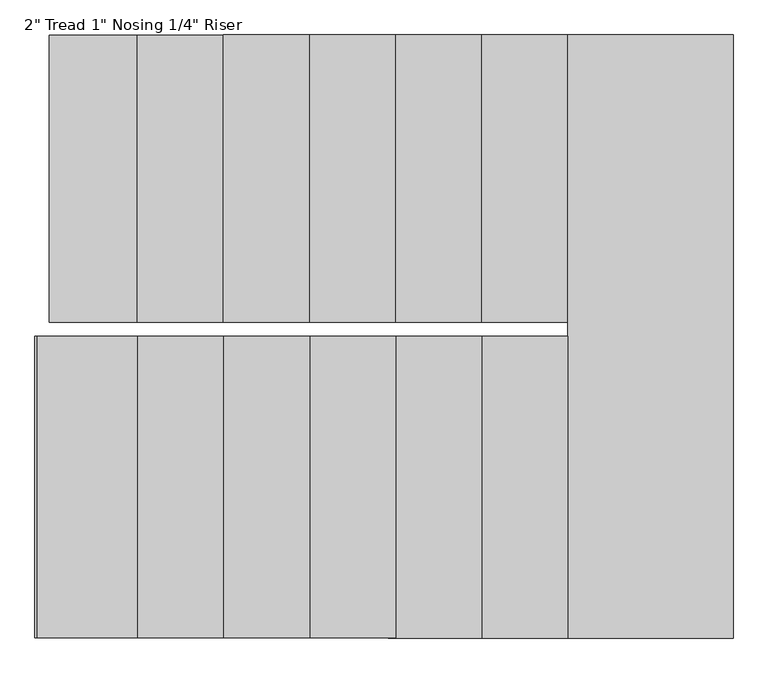
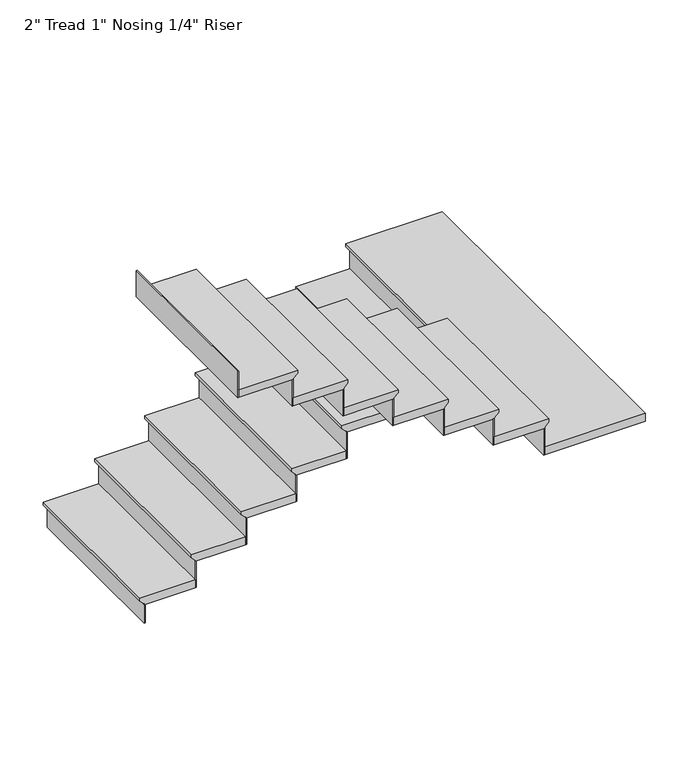
"""IFC4 building model written with IfcOpenShell, lengths in millimetres: stair flight geometry."""

from ifc_helpers import new_model, si_unit, origin, place, context, project, spatial, faceted_brep, source, transform, mapped, element, save


def stair_flight_c67f7d23(model_context):
    return source(origin(), model_context, "Body", "Brep", [
        faceted_brep([(-1167.6638307, -167.7482799, 6551.0833333), (-1167.6638307, -167.7482799, 6570.1333333), (-1167.6638307, 848.2517201, 6570.1333333), (-1167.6638307, 848.2517201, 6551.0833333), (-1142.2638307, -167.7482799, 6525.6833333), (-1142.2638307, 848.2517201, 6525.6833333), (-831.1138307, -167.7482799, 6570.1333333), (-831.1138307, 848.2517201, 6570.1333333), (-1142.2638307, 848.2517201, 6519.3333333), (-831.1138307, 848.2517201, 6519.3333333), (-831.1138307, -167.7482799, 6519.3333333), (-1142.2638307, -167.7482799, 6519.3333333)], [[[0, 1, 2, 3]], [[4, 0, 3, 5]], [[2, 1, 6, 7]], [[8, 9, 10, 11]], [[2, 7, 9, 8, 5, 3]], [[8, 11, 4, 5]], [[6, 1, 0, 4, 11, 10]], [[7, 6, 10, 9]]]),
        faceted_brep([(-1142.2638307, -167.7482799, 6519.3333333), (-1142.2638307, -167.7482799, 6400.8), (-1135.9138307, -167.7482799, 6400.8), (-1135.9138307, -167.7482799, 6519.3333333), (-1142.2638307, 848.2517201, 6519.3333333), (-1135.9138307, 848.2517201, 6519.3333333), (-1135.9138307, 848.2517201, 6400.8), (-1142.2638307, 848.2517201, 6400.8)], [[[0, 1, 2, 3]], [[4, 5, 6, 7]], [[1, 0, 4, 7]], [[2, 1, 7, 6]], [[3, 2, 6, 5]], [[0, 3, 5, 4]]]),
        faceted_brep([(-831.1138307, -167.7482799, 6688.6666667), (-831.1138307, -167.7482799, 6519.3333333), (-824.7638307, -167.7482799, 6519.3333333), (-824.7638307, -167.7482799, 6688.6666667), (-831.1138307, 848.2517201, 6688.6666667), (-824.7638307, 848.2517201, 6688.6666667), (-824.7638307, 848.2517201, 6519.3333333), (-831.1138307, 848.2517201, 6519.3333333)], [[[0, 1, 2, 3]], [[4, 5, 6, 7]], [[1, 0, 4, 7]], [[2, 1, 7, 6]], [[3, 2, 6, 5]], [[0, 3, 5, 4]]]),
        faceted_brep([(-856.5138307, 848.2517201, 6739.4666667), (-856.5138307, -167.7482799, 6739.4666667), (-526.3138307, -167.7482799, 6739.4666667), (-526.3138307, 848.2517201, 6739.4666667), (-831.1138307, 848.2517201, 6688.6666667), (-526.3138307, 848.2517201, 6688.6666667), (-526.3138307, -167.7482799, 6688.6666667), (-831.1138307, -167.7482799, 6688.6666667), (-831.1138307, 848.2517201, 6695.0166667), (-856.5138307, 848.2517201, 6720.4166667), (-831.1138307, -167.7482799, 6695.0166667), (-856.5138307, -167.7482799, 6720.4166667)], [[[0, 1, 2, 3]], [[4, 5, 6, 7]], [[0, 3, 5, 4, 8, 9]], [[4, 7, 10, 8]], [[2, 1, 11, 10, 7, 6]], [[3, 2, 6, 5]], [[11, 1, 0, 9]], [[10, 11, 9, 8]]]),
        faceted_brep([(-526.3138307, -167.7482799, 6858.0), (-526.3138307, -167.7482799, 6688.6666667), (-519.9638307, -167.7482799, 6688.6666667), (-519.9638307, -167.7482799, 6858.0), (-526.3138307, 848.2517201, 6858.0), (-519.9638307, 848.2517201, 6858.0), (-519.9638307, 848.2517201, 6688.6666667), (-526.3138307, 848.2517201, 6688.6666667)], [[[0, 1, 2, 3]], [[4, 5, 6, 7]], [[1, 0, 4, 7]], [[2, 1, 7, 6]], [[3, 2, 6, 5]], [[0, 3, 5, 4]]]),
        faceted_brep([(-551.7138307, 848.2517201, 6908.8), (-551.7138307, -167.7482799, 6908.8), (-221.5138307, -167.7482799, 6908.8), (-221.5138307, 848.2517201, 6908.8), (-526.3138307, 848.2517201, 6858.0), (-221.5138307, 848.2517201, 6858.0), (-221.5138307, -167.7482799, 6858.0), (-526.3138307, -167.7482799, 6858.0), (-526.3138307, 848.2517201, 6864.35), (-551.7138307, 848.2517201, 6889.75), (-526.3138307, -167.7482799, 6864.35), (-551.7138307, -167.7482799, 6889.75)], [[[0, 1, 2, 3]], [[4, 5, 6, 7]], [[0, 3, 5, 4, 8, 9]], [[4, 7, 10, 8]], [[2, 1, 11, 10, 7, 6]], [[3, 2, 6, 5]], [[11, 1, 0, 9]], [[10, 11, 9, 8]]]),
        faceted_brep([(-221.5138307, -167.7482799, 7027.3333333), (-221.5138307, -167.7482799, 6858.0), (-215.1638307, -167.7482799, 6858.0), (-215.1638307, -167.7482799, 7027.3333333), (-221.5138307, 848.2517201, 7027.3333333), (-215.1638307, 848.2517201, 7027.3333333), (-215.1638307, 848.2517201, 6858.0), (-221.5138307, 848.2517201, 6858.0)], [[[0, 1, 2, 3]], [[4, 5, 6, 7]], [[1, 0, 4, 7]], [[2, 1, 7, 6]], [[3, 2, 6, 5]], [[0, 3, 5, 4]]]),
        faceted_brep([(-246.9138307, 848.2517201, 7078.1333333), (-246.9138307, -167.7482799, 7078.1333333), (83.2861693, -167.7482799, 7078.1333333), (83.2861693, 848.2517201, 7078.1333333), (-221.5138307, 848.2517201, 7027.3333333), (83.2861693, 848.2517201, 7027.3333333), (83.2861693, -167.7482799, 7027.3333333), (-221.5138307, -167.7482799, 7027.3333333), (-221.5138307, 848.2517201, 7033.6833333), (-246.9138307, 848.2517201, 7059.0833333), (-221.5138307, -167.7482799, 7033.6833333), (-246.9138307, -167.7482799, 7059.0833333)], [[[0, 1, 2, 3]], [[4, 5, 6, 7]], [[0, 3, 5, 4, 8, 9]], [[4, 7, 10, 8]], [[2, 1, 11, 10, 7, 6]], [[3, 2, 6, 5]], [[11, 1, 0, 9]], [[10, 11, 9, 8]]]),
        faceted_brep([(83.2861693, -167.7482799, 7196.6666667), (83.2861693, -167.7482799, 7027.3333333), (89.6361693, -167.7482799, 7027.3333333), (89.6361693, -167.7482799, 7196.6666667), (83.2861693, 848.2517201, 7196.6666667), (89.6361693, 848.2517201, 7196.6666667), (89.6361693, 848.2517201, 7027.3333333), (83.2861693, 848.2517201, 7027.3333333)], [[[0, 1, 2, 3]], [[4, 5, 6, 7]], [[1, 0, 4, 7]], [[2, 1, 7, 6]], [[3, 2, 6, 5]], [[0, 3, 5, 4]]]),
        faceted_brep([(57.8861693, 848.2517201, 7247.4666667), (57.8861693, -167.7482799, 7247.4666667), (388.0861693, -167.7482799, 7247.4666667), (388.0861693, 848.2517201, 7247.4666667), (83.2861693, 848.2517201, 7196.6666667), (388.0861693, 848.2517201, 7196.6666667), (388.0861693, -167.7482799, 7196.6666667), (83.2861693, -167.7482799, 7196.6666667), (83.2861693, 848.2517201, 7203.0166667), (57.8861693, 848.2517201, 7228.4166667), (83.2861693, -167.7482799, 7203.0166667), (57.8861693, -167.7482799, 7228.4166667)], [[[0, 1, 2, 3]], [[4, 5, 6, 7]], [[0, 3, 5, 4, 8, 9]], [[4, 7, 10, 8]], [[2, 1, 11, 10, 7, 6]], [[3, 2, 6, 5]], [[11, 1, 0, 9]], [[10, 11, 9, 8]]]),
        faceted_brep([(388.0861693, -167.7482799, 7366.0), (388.0861693, -167.7482799, 7196.6666667), (394.4361693, -167.7482799, 7196.6666667), (394.4361693, -167.7482799, 7366.0), (388.0861693, 848.2517201, 7366.0), (394.4361693, 848.2517201, 7366.0), (394.4361693, 848.2517201, 7196.6666667), (388.0861693, 848.2517201, 7196.6666667)], [[[0, 1, 2, 3]], [[4, 5, 6, 7]], [[1, 0, 4, 7]], [[2, 1, 7, 6]], [[3, 2, 6, 5]], [[0, 3, 5, 4]]]),
        faceted_brep([(362.6861693, 848.2517201, 7416.8), (362.6861693, -167.7482799, 7416.8), (692.8861693, -167.7482799, 7416.8), (692.8861693, 848.2517201, 7416.8), (388.0861693, 848.2517201, 7366.0), (692.8861693, 848.2517201, 7366.0), (692.8861693, -167.7482799, 7366.0), (388.0861693, -167.7482799, 7366.0), (388.0861693, 848.2517201, 7372.35), (362.6861693, 848.2517201, 7397.75), (388.0861693, -167.7482799, 7372.35), (362.6861693, -167.7482799, 7397.75)], [[[0, 1, 2, 3]], [[4, 5, 6, 7]], [[0, 3, 5, 4, 8, 9]], [[4, 7, 10, 8]], [[2, 1, 11, 10, 7, 6]], [[3, 2, 6, 5]], [[11, 1, 0, 9]], [[10, 11, 9, 8]]]),
        faceted_brep([(692.8861693, -167.7482799, 7535.3333333), (692.8861693, -167.7482799, 7366.0), (699.2361693, -167.7482799, 7366.0), (699.2361693, -167.7482799, 7535.3333333), (692.8861693, 848.2517201, 7535.3333333), (699.2361693, 848.2517201, 7535.3333333), (699.2361693, 848.2517201, 7366.0), (692.8861693, 848.2517201, 7366.0)], [[[0, 1, 2, 3]], [[4, 5, 6, 7]], [[1, 0, 4, 7]], [[2, 1, 7, 6]], [[3, 2, 6, 5]], [[0, 3, 5, 4]]]),
        faceted_brep([(642.0861693, -1285.3482799, 7586.1333333), (1251.6861693, -1285.3482799, 7586.1333333), (1251.6861693, 848.2517201, 7586.1333333), (667.4861693, 848.2517201, 7586.1333333), (667.4861693, -218.5482799, 7586.1333333), (642.0861693, -218.5482799, 7586.1333333), (1251.6861693, -1285.3482799, 7535.3333333), (642.0861693, -1285.3482799, 7535.3333333), (642.0861693, -218.5482799, 7535.3333333), (667.4861693, -218.5482799, 7535.3333333), (667.4861693, -167.7482799, 7535.3333333), (692.8861693, -167.7482799, 7535.3333333), (692.8861693, 848.2517201, 7535.3333333), (1251.6861693, 848.2517201, 7535.3333333), (692.8861693, 848.2517201, 7541.6833333), (667.4861693, 848.2517201, 7567.0833333), (692.8861693, -167.7482799, 7541.6833333), (667.4861693, -167.7482799, 7567.0833333)], [[[0, 1, 2, 3, 4, 5]], [[6, 7, 8, 9, 10, 11, 12, 13]], [[1, 0, 7, 6]], [[2, 1, 6, 13]], [[3, 2, 13, 12, 14, 15]], [[12, 11, 16, 14]], [[11, 10, 17, 16]], [[4, 3, 15, 17, 10, 9]], [[5, 4, 9, 8]], [[0, 5, 8, 7]], [[15, 14, 16, 17]]]),
        faceted_brep([(642.0861693, -218.5482799, 7704.6666667), (642.0861693, -218.5482799, 7535.3333333), (635.7361693, -218.5482799, 7535.3333333), (635.7361693, -218.5482799, 7704.6666667), (642.0861693, -1285.3482799, 7704.6666667), (635.7361693, -1285.3482799, 7704.6666667), (635.7361693, -1285.3482799, 7535.3333333), (642.0861693, -1285.3482799, 7535.3333333)], [[[0, 1, 2, 3]], [[4, 5, 6, 7]], [[1, 0, 4, 7]], [[2, 1, 7, 6]], [[3, 2, 6, 5]], [[0, 3, 5, 4]]]),
        faceted_brep([(667.4861693, -1285.3482799, 7755.4666667), (667.4861693, -218.5482799, 7755.4666667), (337.2861693, -218.5482799, 7755.4666667), (337.2861693, -1285.3482799, 7755.4666667), (642.0861693, -1285.3482799, 7704.6666667), (337.2861693, -1285.3482799, 7704.6666667), (337.2861693, -218.5482799, 7704.6666667), (642.0861693, -218.5482799, 7704.6666667), (642.0861693, -1285.3482799, 7711.0166667), (667.4861693, -1285.3482799, 7736.4166667), (642.0861693, -218.5482799, 7711.0166667), (667.4861693, -218.5482799, 7736.4166667)], [[[0, 1, 2, 3]], [[4, 5, 6, 7]], [[0, 3, 5, 4, 8, 9]], [[4, 7, 10, 8]], [[2, 1, 11, 10, 7, 6]], [[3, 2, 6, 5]], [[11, 1, 0, 9]], [[10, 11, 9, 8]]]),
        faceted_brep([(337.2861693, -218.5482799, 7874.0), (337.2861693, -218.5482799, 7704.6666667), (330.9361693, -218.5482799, 7704.6666667), (330.9361693, -218.5482799, 7874.0), (337.2861693, -1285.3482799, 7874.0), (330.9361693, -1285.3482799, 7874.0), (330.9361693, -1285.3482799, 7704.6666667), (337.2861693, -1285.3482799, 7704.6666667)], [[[0, 1, 2, 3]], [[4, 5, 6, 7]], [[1, 0, 4, 7]], [[2, 1, 7, 6]], [[3, 2, 6, 5]], [[0, 3, 5, 4]]]),
        faceted_brep([(362.6861693, -1285.3482799, 7924.8), (362.6861693, -218.5482799, 7924.8), (32.4861693, -218.5482799, 7924.8), (32.4861693, -1285.3482799, 7924.8), (337.2861693, -1285.3482799, 7874.0), (32.4861693, -1285.3482799, 7874.0), (32.4861693, -218.5482799, 7874.0), (337.2861693, -218.5482799, 7874.0), (337.2861693, -1285.3482799, 7880.35), (362.6861693, -1285.3482799, 7905.75), (337.2861693, -218.5482799, 7880.35), (362.6861693, -218.5482799, 7905.75)], [[[0, 1, 2, 3]], [[4, 5, 6, 7]], [[0, 3, 5, 4, 8, 9]], [[4, 7, 10, 8]], [[2, 1, 11, 10, 7, 6]], [[3, 2, 6, 5]], [[11, 1, 0, 9]], [[10, 11, 9, 8]]]),
        faceted_brep([(32.4861693, -218.5482799, 8043.3333333), (32.4861693, -218.5482799, 7874.0), (26.1361693, -218.5482799, 7874.0), (26.1361693, -218.5482799, 8043.3333333), (32.4861693, -1285.3482799, 8043.3333333), (26.1361693, -1285.3482799, 8043.3333333), (26.1361693, -1285.3482799, 7874.0), (32.4861693, -1285.3482799, 7874.0)], [[[0, 1, 2, 3]], [[4, 5, 6, 7]], [[1, 0, 4, 7]], [[2, 1, 7, 6]], [[3, 2, 6, 5]], [[0, 3, 5, 4]]]),
        faceted_brep([(57.8861693, -1285.3482799, 8094.1333333), (57.8861693, -218.5482799, 8094.1333333), (-272.3138307, -218.5482799, 8094.1333333), (-272.3138307, -1285.3482799, 8094.1333333), (32.4861693, -1285.3482799, 8043.3333333), (-272.3138307, -1285.3482799, 8043.3333333), (-272.3138307, -218.5482799, 8043.3333333), (32.4861693, -218.5482799, 8043.3333333), (32.4861693, -1285.3482799, 8049.6833333), (57.8861693, -1285.3482799, 8075.0833333), (32.4861693, -218.5482799, 8049.6833333), (57.8861693, -218.5482799, 8075.0833333)], [[[0, 1, 2, 3]], [[4, 5, 6, 7]], [[0, 3, 5, 4, 8, 9]], [[4, 7, 10, 8]], [[2, 1, 11, 10, 7, 6]], [[3, 2, 6, 5]], [[11, 1, 0, 9]], [[10, 11, 9, 8]]]),
        faceted_brep([(-272.3138307, -218.5482799, 8212.6666667), (-272.3138307, -218.5482799, 8043.3333333), (-278.6638307, -218.5482799, 8043.3333333), (-278.6638307, -218.5482799, 8212.6666667), (-272.3138307, -1285.3482799, 8212.6666667), (-278.6638307, -1285.3482799, 8212.6666667), (-278.6638307, -1285.3482799, 8043.3333333), (-272.3138307, -1285.3482799, 8043.3333333)], [[[0, 1, 2, 3]], [[4, 5, 6, 7]], [[1, 0, 4, 7]], [[2, 1, 7, 6]], [[3, 2, 6, 5]], [[0, 3, 5, 4]]]),
        faceted_brep([(-246.9138307, -1285.3482799, 8263.4666667), (-246.9138307, -218.5482799, 8263.4666667), (-577.1138307, -218.5482799, 8263.4666667), (-577.1138307, -1285.3482799, 8263.4666667), (-272.3138307, -1285.3482799, 8212.6666667), (-577.1138307, -1285.3482799, 8212.6666667), (-577.1138307, -218.5482799, 8212.6666667), (-272.3138307, -218.5482799, 8212.6666667), (-272.3138307, -1285.3482799, 8219.0166667), (-246.9138307, -1285.3482799, 8244.4166667), (-272.3138307, -218.5482799, 8219.0166667), (-246.9138307, -218.5482799, 8244.4166667)], [[[0, 1, 2, 3]], [[4, 5, 6, 7]], [[0, 3, 5, 4, 8, 9]], [[4, 7, 10, 8]], [[2, 1, 11, 10, 7, 6]], [[3, 2, 6, 5]], [[11, 1, 0, 9]], [[10, 11, 9, 8]]]),
        faceted_brep([(-577.1138307, -218.5482799, 8382.0), (-577.1138307, -218.5482799, 8212.6666667), (-583.4638307, -218.5482799, 8212.6666667), (-583.4638307, -218.5482799, 8382.0), (-577.1138307, -1285.3482799, 8382.0), (-583.4638307, -1285.3482799, 8382.0), (-583.4638307, -1285.3482799, 8212.6666667), (-577.1138307, -1285.3482799, 8212.6666667)], [[[0, 1, 2, 3]], [[4, 5, 6, 7]], [[1, 0, 4, 7]], [[2, 1, 7, 6]], [[3, 2, 6, 5]], [[0, 3, 5, 4]]]),
        faceted_brep([(-551.7138307, -1285.3482799, 8432.8), (-551.7138307, -218.5482799, 8432.8), (-881.9138307, -218.5482799, 8432.8), (-881.9138307, -1285.3482799, 8432.8), (-577.1138307, -1285.3482799, 8382.0), (-881.9138307, -1285.3482799, 8382.0), (-881.9138307, -218.5482799, 8382.0), (-577.1138307, -218.5482799, 8382.0), (-577.1138307, -1285.3482799, 8388.35), (-551.7138307, -1285.3482799, 8413.75), (-577.1138307, -218.5482799, 8388.35), (-551.7138307, -218.5482799, 8413.75)], [[[0, 1, 2, 3]], [[4, 5, 6, 7]], [[0, 3, 5, 4, 8, 9]], [[4, 7, 10, 8]], [[2, 1, 11, 10, 7, 6]], [[3, 2, 6, 5]], [[11, 1, 0, 9]], [[10, 11, 9, 8]]]),
        faceted_brep([(-881.9138307, -218.5482799, 8551.3333333), (-881.9138307, -218.5482799, 8382.0), (-888.2638307, -218.5482799, 8382.0), (-888.2638307, -218.5482799, 8551.3333333), (-881.9138307, -1285.3482799, 8551.3333333), (-888.2638307, -1285.3482799, 8551.3333333), (-888.2638307, -1285.3482799, 8382.0), (-881.9138307, -1285.3482799, 8382.0)], [[[0, 1, 2, 3]], [[4, 5, 6, 7]], [[1, 0, 4, 7]], [[2, 1, 7, 6]], [[3, 2, 6, 5]], [[0, 3, 5, 4]]]),
        faceted_brep([(-1212.1138307, -218.5482799, 8720.6666667), (-1212.1138307, -218.5482799, 8551.3333333), (-1218.4638307, -218.5482799, 8551.3333333), (-1218.4638307, -218.5482799, 8720.6666667), (-1212.1138307, -1285.3482799, 8720.6666667), (-1218.4638307, -1285.3482799, 8720.6666667), (-1218.4638307, -1285.3482799, 8551.3333333), (-1212.1138307, -1285.3482799, 8551.3333333)], [[[0, 1, 2, 3]], [[4, 5, 6, 7]], [[1, 0, 4, 7]], [[2, 1, 7, 6]], [[3, 2, 6, 5]], [[0, 3, 5, 4]]]),
        faceted_brep([(-856.5138307, -1285.3482799, 8602.1333333), (-856.5138307, -218.5482799, 8602.1333333), (-1212.1138307, -218.5482799, 8602.1333333), (-1212.1138307, -1285.3482799, 8602.1333333), (-881.9138307, -1285.3482799, 8551.3333333), (-1212.1138307, -1285.3482799, 8551.3333333), (-1212.1138307, -218.5482799, 8551.3333333), (-881.9138307, -218.5482799, 8551.3333333), (-881.9138307, -1285.3482799, 8557.6833333), (-856.5138307, -1285.3482799, 8583.0833333), (-881.9138307, -218.5482799, 8557.6833333), (-856.5138307, -218.5482799, 8583.0833333)], [[[0, 1, 2, 3]], [[4, 5, 6, 7]], [[0, 3, 5, 4, 8, 9]], [[4, 7, 10, 8]], [[2, 1, 11, 10, 7, 6]], [[3, 2, 6, 5]], [[11, 1, 0, 9]], [[10, 11, 9, 8]]]),
    ])


if __name__ == "__main__":
    model = new_model("IFC4")
    model_context = context("Model", 3, world=origin())
    ifc_project = project(units=[si_unit("LENGTHUNIT", "METRE", prefix="MILLI")], contexts=[model_context])
    site = spatial("IfcSite", under=ifc_project)
    building = spatial("IfcBuilding", under=site)
    placement = place(None, origin())
    stair_flight_shape = stair_flight_c67f7d23(model_context)
    element("IfcStairFlight", 1, ObjectType="2\" Tread 1\" Nosing 1/4\" Riser", at=placement, inside=building, context=model_context, shape_type="MappedRepresentation", body=[
        mapped(stair_flight_shape, transform((0.0, 0.0, 0.0), x_axis=(1.0, 0.0, 0.0), y_axis=(0.0, 1.0, 0.0), z_axis=(0.0, 0.0, 1.0))),
    ])
    save(model, "model.ifc")
